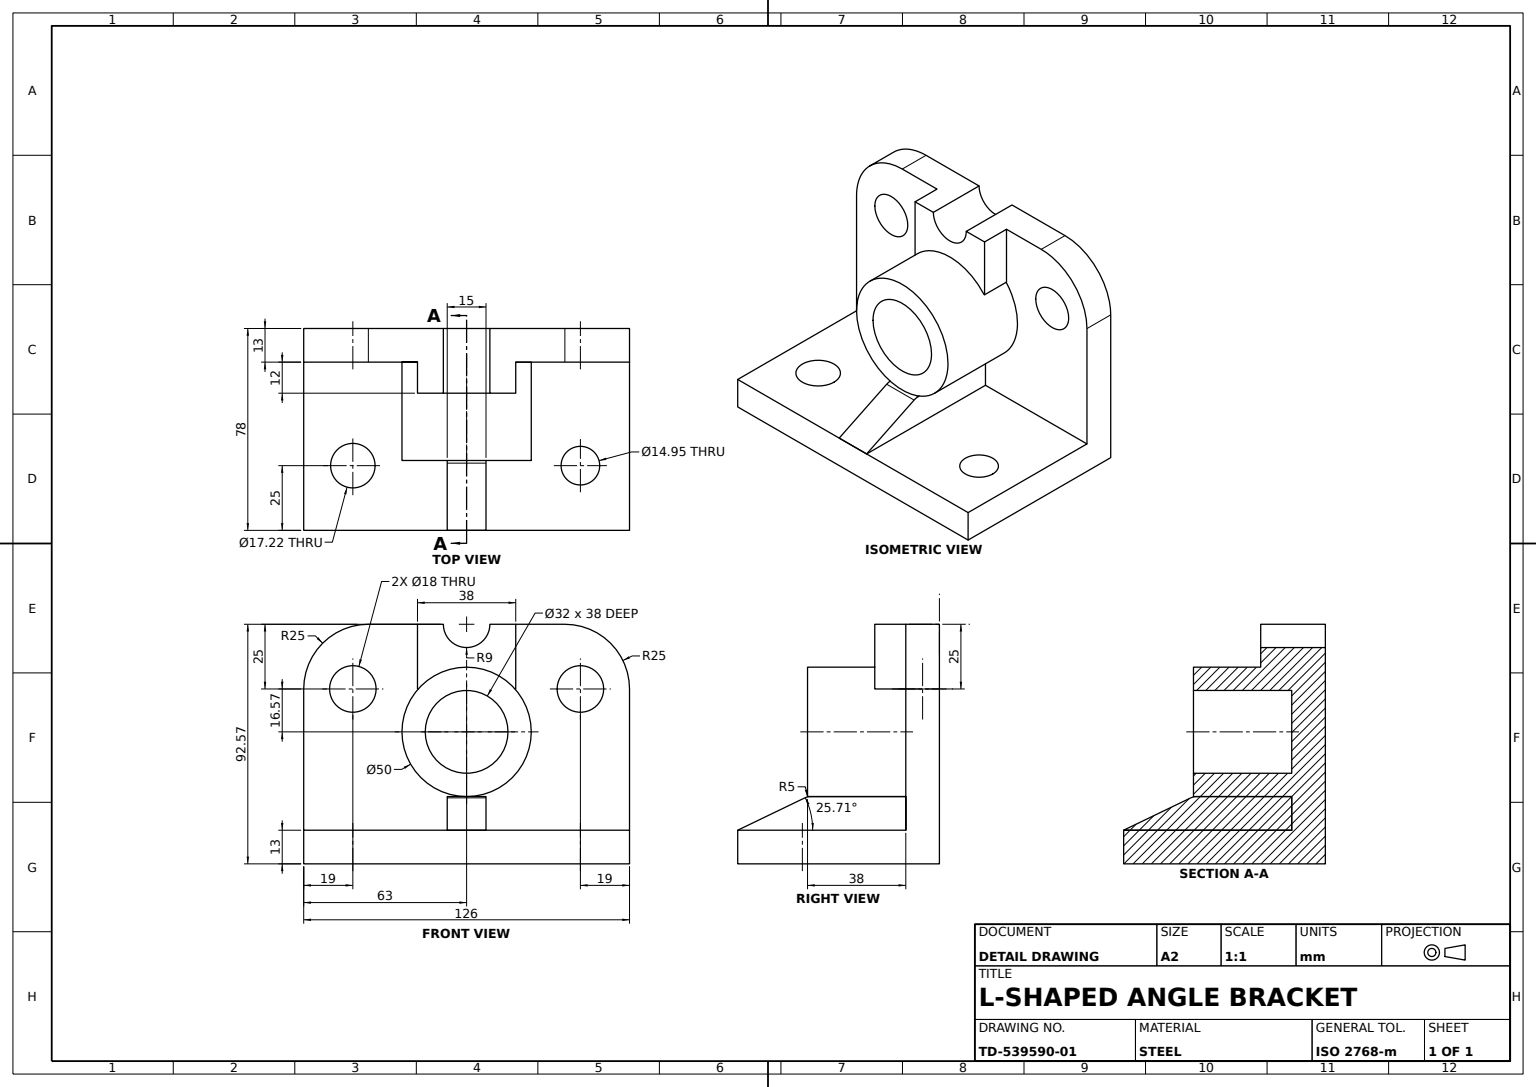
SolidWorks part; units mm, degrees
material "Plain Carbon Steel"
ref_plane "Front Plane" through (0, 0, 0) normal (0, 0, 1) x (1, 0, 0)
ref_plane "Top Plane" through (0, 0, 0) normal (0, 1, 0) x (1, 0, 0)
ref_plane "Right Plane" through (0, 0, 0) normal (1, 0, 0) x (0, 0, -1)
sketch "Base Plate Sketch" plane through (0, 0, 0) normal (0, 1, 0) x (1, 0, 0)
  line L1 (-39, -63) -> (39, -63)
  line L2 (-39, -63) -> (-39, 63)
  line L3 (-39, 63) -> (39, 63)
  line L4 (39, -63) -> (39, 63)
  line L5 (-39, -63) -> (39, 63) construction
  line L6 (-39, 63) -> (39, -63) construction
  point P0 (0, 0)
  dimension "D1" = 126
  dimension "D2" = 78
extrude "Base Plate 126x78x13" add sketch "Base Plate Sketch" along normal blind 13
sketch "Upright Plate Sketch" plane through (-39, 0, 0) normal (-1, 0, 0) x (0, 0, 1)
  line L0 (63, 0) -> (63, 92.5743)
  line L1 (63, 92.5743) -> (-63, 92.5743)
  line L2 (-63, 92.5743) -> (-63, 0)
  line L3 (-63, 0) -> (63, 0)
  line L4 (-63, 0) -> (63, 0) construction
  dimension "D1" = 92.5743
extrude "Upright Plate" add sketch "Upright Plate Sketch" against normal blind 13
fillet "Upright Corner Fillet R25 A" radius 25 1 edges at (-32.5, 92.5743, 63)
fillet "Upright Corner Fillet R25 B" radius 25 1 edges at (-32.5, 92.5743, -63)
sketch "Upright Top Block Sketch" plane through (-39, 0, 0) normal (-1, 0, 0) x (0, 0, 1)
  line L0 (38, 92.5743) -> (-38, 92.5743) construction
  line L1 (-9, 92.5743) -> (-19, 92.5743)
  line L2 (-19, 92.5743) -> (-19, 67.5743)
  line L3 (-19, 67.5743) -> (19, 67.5743)
  line L4 (19, 67.5743) -> (19, 92.5743)
  line L5 (19, 92.5743) -> (9, 92.5743)
  circle A0 centre (0, 92.5743) radius 9
  line M4 (38, 92.5743) -> (-38, 92.5743)
  dimension "D1" = 10
  dimension "D3" = 18
  dimension "D2" = 10
  dimension "D4" = 25
extrude "Upright Top Block" add sketch "Upright Top Block Sketch" against normal blind 25 contours A0 L2 L3 L4 M4
sketch "Top Notch Sketch" plane through (-39, 0, 0) normal (-1, 0, 0) x (0, 0, 1)
  line L0 (38, 92.5743) -> (-38, 92.5743) construction
  circle A0 centre (0, 92.5743) radius 9
  dimension "D1" = 18
extrude "Top Notch Ø18" cut sketch "Top Notch Sketch" against normal blind 25
sketch "Upright Holes Sketch" plane through (-26, 0, 0) normal (1, 0, 0) x (0, 0, -1)
  line L0 (-38, 92.5743) -> (-19, 92.5743) construction
  line L2 (-63, 13) -> (-63, 67.5743) construction
  line L3 (19, 92.5743) -> (38, 92.5743) construction
  line L4 (63, 67.5743) -> (63, 13) construction
  circle A0 centre (-44, 67.5743) radius 9
  circle A1 centre (44, 67.5743) radius 9
  dimension "D1" = 18
  dimension "D2" = 18
  dimension "D3" = 25
  dimension "D4" = 19
  dimension "D5" = 25
  dimension "D6" = 19
extrude "Upright Holes 2x" cut sketch "Upright Holes Sketch" against normal blind 25
sketch "Base Holes Sketch" plane through (0, 13, 0) normal (0, 1, 0) x (1, 0, 0)
  line L0 (39, 63) -> (-26, 63) construction
  line L1 (39, -63) -> (39, 63) construction
  line L2 (-26, -63) -> (39, -63) construction
  circle A0 centre (14, 44) radius 7.4725
  circle A1 centre (14, -44) radius 8.6091
  dimension "D1" = 19
  dimension "D5" = 14.9451
  dimension "D6" = 17.2182
  dimension "D2" = 25
  dimension "D3" = 19
  dimension "D4" = 25
extrude "Base Mounting Holes 2x" cut sketch "Base Holes Sketch" against normal blind 25
sketch "Hub Boss Sketch" plane through (-26, 0, 0) normal (1, 0, 0) x (0, 0, -1)
  line L0 (-19, 67.5743) -> (-19, 92.5743) construction
  line L1 (19, 67.5743) -> (-19, 67.5743) construction
  circle A0 centre (0, 51) radius 25
  dimension "D2" = 19
  dimension "D1" = 50
  dimension "D3" = 16.5743
extrude "Hub Boss" add sketch "Hub Boss Sketch" along normal blind 38
sketch "Hub Bore Sketch" plane through (12, 0, 0) normal (1, 0, 0) x (0, 0, -1)
  circle A0 centre (0, 51) radius 16
  dimension "D1" = 32
extrude "Hub Bore" cut sketch "Hub Bore Sketch" against normal blind 38
sketch "Gusset Rib Sketch" plane through (0, 0, 0) normal (0, 0, 1) x (1, 0, 0)
  line L0 (-26, 26) -> (12, 26) construction
  line L1 (-26, 26) -> (12, 26)
  line L2 (-26, 26) -> (-26, 13)
  line L3 (-26, 13) -> (39, 13)
  line L4 (39, 13) -> (12, 26)
extrude "Gusset Rib" add sketch "Gusset Rib Sketch" along normal mid plane 15 separate body
fillet "Gusset Rib Fillet R5" radius 5 1 edges at (12, 26, 0)
